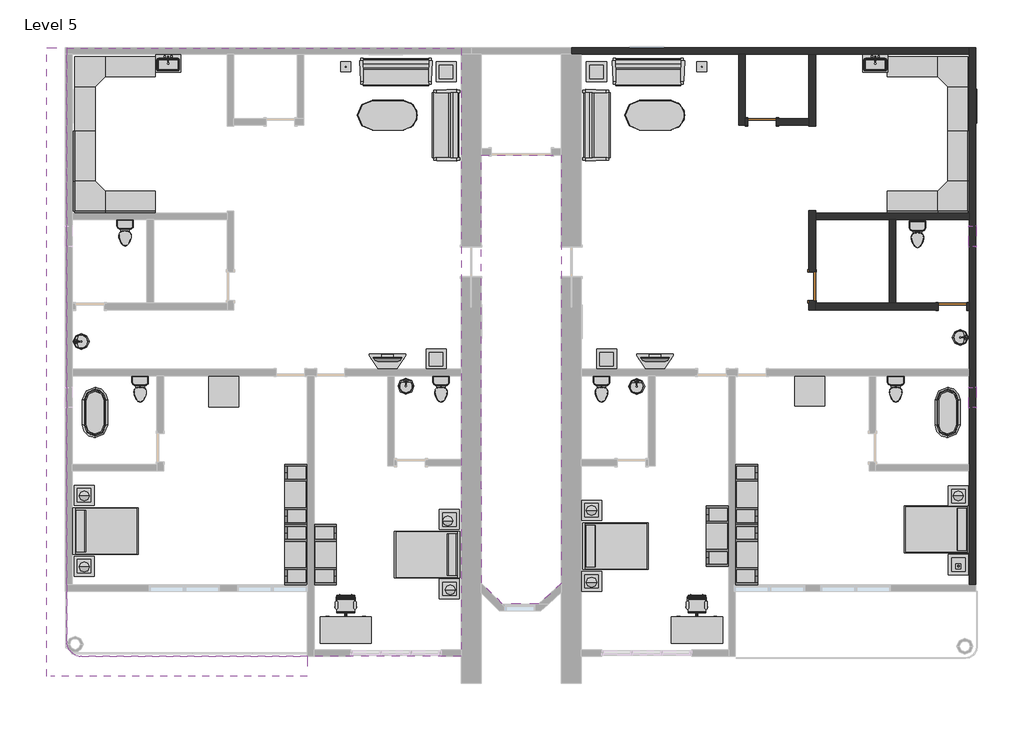
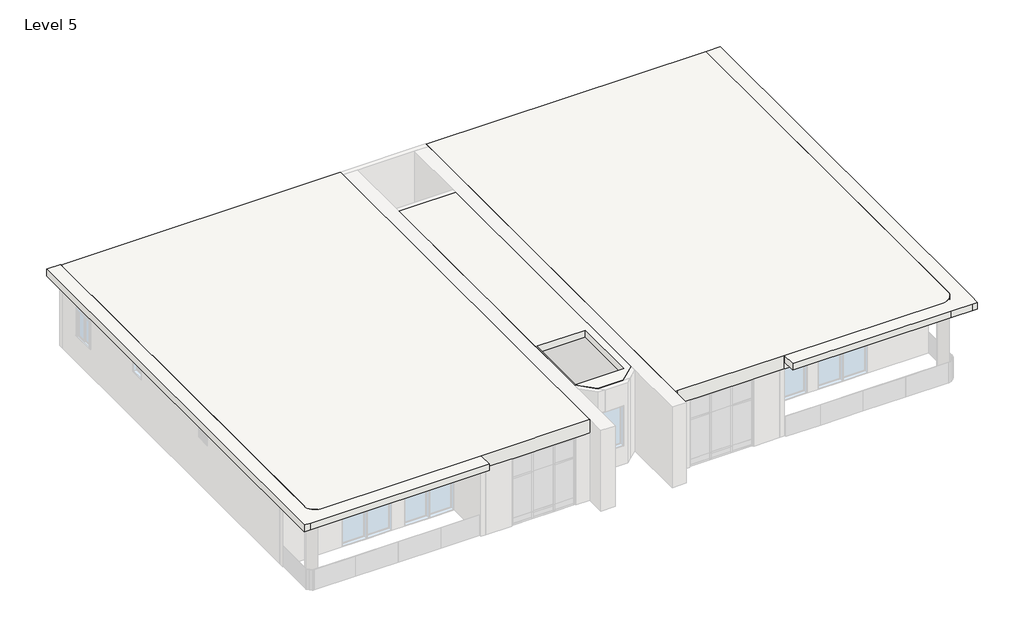
# One storey, part 3 of 3: 42 furniture elements, 14 flow terminals, 10 light fixtures, 9 walls, 3 doors, 3 slabs, 3 windows.
# Revit data of these elements (continued)
# Elements 40, 41 (IfcFurniture, "TV Stand : TV Stand")
#   Phase Created = New Construction
#   Materials on its faces: "Melamine - Gray", "Glass - Shelves"
# Elements 42, 43, 44, 45, 46, 47, 48, 49, 50, 51, 52, 53 (IfcFurniture, "Table-Coffee : 24\" x 24\" x 24\"")
#   Phase Created = New Construction
#   Materials on its faces: "Glass - Clear, Grey"
# Elements 54, 55 (IfcFurniture, "Table-Dining Oval : 36\" x 72\"")
#   Phase Created = New Construction
#   Materials on its faces: "Steel, Chrome Plated", "Glass - Clear, Grey"
# Elements 56, 57 (IfcFurniture, "Table-Rectangular : 36\" x 36\"")
#   Phase Created = New Construction
#   Materials on its faces: "Birch"
# Elements 58, 59 (IfcFurniture, "Work Station Cubicle : 96\" x 96\"")
#   Phase Created = New Construction
#   Materials on its faces: "Textile - Light Gray", "Laminate, Ivory, Matte"
# Element 60 (IfcLightFixture, "100W - 120V")
#   Mark = "64"
#   Phase Created = New Construction
#   Materials on its faces: "Steel, Chrome Plated", "Glass, Frosted"
# Element 61 (IfcLightFixture, "100W - 120V")
#   Mark = "65"
#   Phase Created = New Construction
#   Materials on its faces: "Steel, Chrome Plated", "Glass, Frosted"
# Element 62 (IfcLightFixture, "Table Lamp - Hemispheric : 60W - 120V")
#   Mark = "66"
#   Phase Created = New Construction
#   Materials on its faces: "Steel, Chrome Plated", "Glass, Frosted", "Birch"
# Element 63 (IfcLightFixture, "Table Lamp - Hemispheric : 60W - 120V")
#   Mark = "67"
#   Phase Created = New Construction
#   Materials on its faces: "Steel, Chrome Plated", "Glass, Frosted", "Birch"
# Element 64 (IfcLightFixture, "Table Lamp - Hemispheric : 60W - 120V")
#   Mark = "68"
#   Phase Created = New Construction
#   Materials on its faces: "Steel, Chrome Plated", "Glass, Frosted", "Birch"
# Element 65 (IfcLightFixture, "Table Lamp - Hemispheric : 60W - 120V")
#   Mark = "69"
#   Phase Created = New Construction
#   Materials on its faces: "Steel, Chrome Plated", "Glass, Frosted", "Birch"
# Element 66 (IfcLightFixture, "Table Lamp - Hemispheric : 60W - 120V")
#   Mark = "70"
#   Phase Created = New Construction
#   Materials on its faces: "Steel, Chrome Plated", "Glass, Frosted", "Birch"
# Element 67 (IfcLightFixture, "Table Lamp - Hemispheric : 60W - 120V")
#   Mark = "71"
#   Phase Created = New Construction
#   Materials on its faces: "Steel, Chrome Plated", "Glass, Frosted", "Birch"
# Element 68 (IfcLightFixture, "Table Lamp - Hemispheric : 60W - 120V")
#   Mark = "72"
#   Phase Created = New Construction
#   Materials on its faces: "Steel, Chrome Plated", "Glass, Frosted", "Birch"
# Element 69 (IfcLightFixture, "Table Lamp - Hemispheric : 60W - 120V")
#   Mark = "73"
#   Phase Created = New Construction
#   Materials on its faces: "Steel, Chrome Plated", "Glass, Frosted", "Birch"
# Element 70 (IfcSlab, "Generic - 12\" cream")
#   Height Offset From Level = 12' - 0"
#   Phase Created = New Construction
#   Materials on its faces: "Parking Stripe"
# Element 71 (IfcSlab, "Generic - 12\" white")
#   built-in parameter 1001955 = 3.14159 (stored number, unit not read)
#   Height Offset From Level = 12' - 0"
#   Phase Created = New Construction
#   Materials on its faces: "Door - Frame"
# Element 72 (IfcSlab, "Generic - 12\" white")
#   Height Offset From Level = 12' - 0"
#   Phase Created = New Construction
#   Materials on its faces: "Door - Frame"
# Elements 73, 74, 75, 76, 77, 78, 79, 80 (IfcWall, "Generic - 8\" cream")
#   Top Offset = 0' - 0"
#   Base Offset = 0' - 0"
#   Unconnected Height = 10' - 0"
#   wall height = 10' - 0"
#   Phase Created = New Construction
#   Base Constraint = Level 5
#   Materials on its faces: "Parking Stripe"
# Element 81 (IfcWall, "Generic - 8\" white")
#   Top Offset = 0' - 0"
#   Base Offset = 0' - 0"
#   Unconnected Height = 10' - 0"
#   wall height = 10' - 0"
#   Phase Created = New Construction
#   Base Constraint = Level 5
#   Materials on its faces: "Door - Frame", "Parking Stripe"
# Element 82 (IfcWindow, "Louvers with Trim : 24\" x 24\"")
#   Mark = "129"
#   Phase Created = New Construction
#   Materials on its faces: "Glass", "Iron, Ductile"
# Element 83 (IfcWindow, "Louvers with Trim : 24\" x 24\"")
#   Mark = "130"
#   Phase Created = New Construction
#   Materials on its faces: "Glass", "Iron, Ductile"
# Element 84 (IfcWindow, "Slider with Trim : 36\" x 48\"")
#   Mark = "126"
#   Phase Created = New Construction
#   Materials on its faces: "Iron, Ductile", "Glass"
# Materials
#   "Wood - Birch - Solid Stained Light Low Gloss": class "Wood", colour RGB 210 159 95, transparency 0, Cost = 0
#   "Paint - Sienna": colour RGB 118 70 51, transparency 0, Cost = 0
#   "Steel, Polished": class "Metal", colour RGB 57 57 57, transparency 0, Description = "Polished steel", Cost = 0
#   "Porcelain, Linen": class "Ceramic", colour RGB 249 239 230, transparency 0, Description = "Porcelain, linen", Cost = 0
#   "Laminate, Linen, Matte": class "Plastic", colour RGB 249 239 230, transparency 0, Description = "Plastic Laminate - Linen, Matte", Cost = 0
#   "Porcelain, Ivory": class "Ceramic", colour RGB 247 247 239, transparency 0, Description = "Porcelain, ivory", Cost = 0
#   "Laminate, Ivory, Matte": class "Plastic", colour RGB 247 247 239, transparency 0, Description = "Plastic Laminate - Ivory, Matte", Cost = 0
#   "Birch": class "Wood", colour RGB 224 178 126, transparency 0, Description = "Betula Alleghaniensis", Cost = 0
#   "Linen, White": class "Textile", colour RGB 247 247 239, transparency 0, Description = "Linen, white", Cost = 0
#   "Plastic, Opaque Black": class "Plastic", colour RGB 0 0 0, transparency 0.7, Description = "Plastic, generic, opaque black", Cost = 0
#   "Textile - Slate Blue": class "Fabric", colour RGB 98 102 118, transparency 0
#   "Steel, Chrome Plated": class "Metal", colour RGB 17 17 17, transparency 0, Description = "Chromiuim plated steel", Cost = 0
#   "Cherry": class "Wood", colour RGB 226 177 128, transparency 0, Description = "Prunus Serotina", Cost = 0
#   "Linen, Beige": class "Textile", colour RGB 249 239 230, transparency 0, Description = "Linen, beige", Cost = 0
#   "Melamine - Gray": class "Wood", colour RGB 49 49 49, transparency 0
#   "Glass - Clear, Grey": class "Glass", colour RGB 252 255 255, transparency 0.64
#   "Textile - Light Gray": class "Fabric", colour RGB 204 204 204, transparency 0
#   "Glass, Frosted": class "Glass", colour RGB 250 244 225, transparency 0.55, Description = "physical material", Cost = 0
#   "Parking Stripe": class "Paint", colour RGB 250 250 91, transparency 0, Cost = 0
#   "Door - Frame": colour RGB 118 70 51, transparency 0, Cost = 0
#   "Iron, Ductile": class "Metal", colour RGB 0 0 0, transparency 0, Description = "Ductile cast iron", Cost = 0
#   "Glass": class "Glass", colour RGB 0 128 192, transparency 0.75, Description = "Soda Lime Glass", Cost = 0
#   "TV - Black": colour RGB 49 49 49, transparency 0
#   "TV - Glass": colour RGB 157 157 157, transparency 0.9
#   "TV - Screen": colour RGB 0 0 0, transparency 0
#   "Glass - Shelves": class "Glass", colour RGB 167 167 167, transparency 0.9
